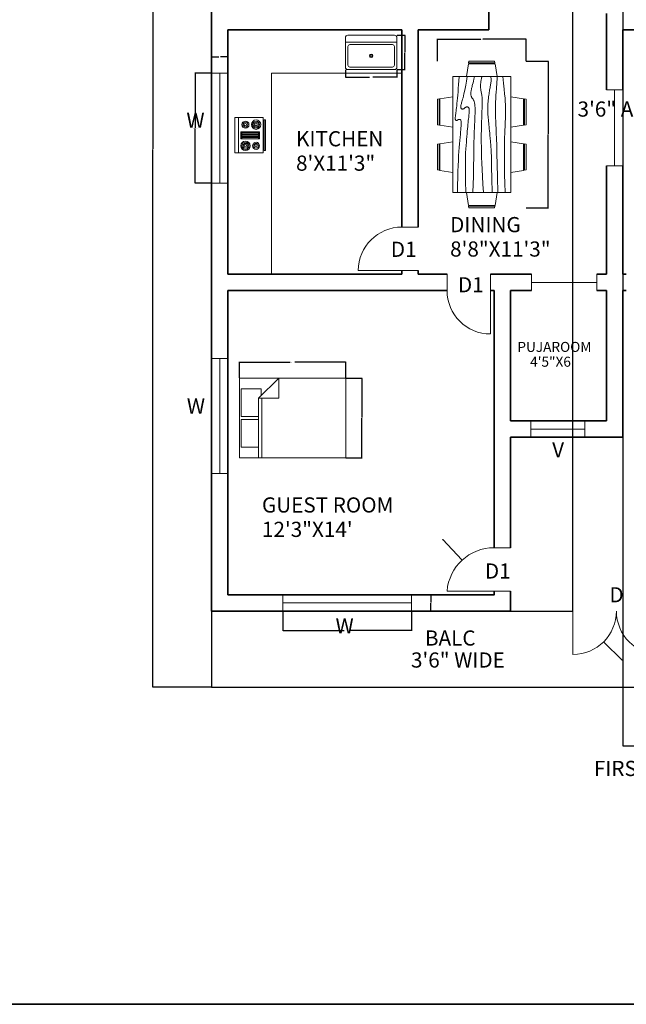
# Model space of a CAD drawing. Units: feet. Extents: x 1654 to 2985, y 1348 to 2230.
# Tile 41 of 53: x 2320 to 2655, y 1348 to 1892. Entities that reach past the tile are written whole.
import ezdxf

# ---------------------------------------------------------------- set-up
doc = ezdxf.new("R2010")
doc.units = ezdxf.units.FT
for name, color, linetype, lineweight in [('A-ANNO-DIMS', 2, 'Continuous', 18), ('A-ANNO-TEXT', 7, 'Continuous', 18), ('A-ANNO-TITL', 7, 'Continuous', 35), ('A-ANNO-TTLB', 7, 'Continuous', 35), ('A-AREA-IDEN', 7, 'Continuous', 18), ('A-DOOR', 3, 'Continuous', 18), ('A-EQPM', 9, 'Continuous', 18), ('A-FLOR', 7, 'Continuous', 25), ('A-FLOR-CASE', 8, 'Continuous', 18), ('A-FLOR-FIXT', 8, 'Continuous', 18), ('A-FURN', 8, 'Continuous', 13), ('A-GLAZ', 4, 'Continuous', 18), ('A-WALL', 7, 'Continuous', 35), ('A-WALL-OPEN', 4, 'Continuous', 18)]:
    doc.layers.add(name, color=color, linetype=linetype, lineweight=lineweight)
doc.styles.get("Standard").update_dxf_attribs({"font": 'arial.ttf'})
doc.dimstyles.get("Standard").update_dxf_attribs({"dimtxt": 0.18, "dimasz": 0.18, "dimexe": 0.18, "dimexo": 0.0625, "dimgap": 0.09, "dimtad": 0, "dimtih": 1, "dimtoh": 1, "dimdec": 4, "dimzin": 0, "dimdsep": 46, "dimtxsty": 'Standard', "dimcen": 0.09, "dimadec": 0, "dimazin": 0, "dimtfac": 1, "dimtdec": 4, "dimtofl": 0, "dimtmove": 0, "dimatfit": 3, "dimfxl": 1, "dimtolj": 1, "dimtzin": 0, "dimarcsym": 0})

# ---------------------------------------------------------------- blocks, each defined once
blk = doc.blocks.new('Dining Set - 36 x 72 in.')
for p, q in [((-22.2343, 26.00059), (-23.4847, 17.99762)), ((-22.2304, 26), (-5.7608, 26)), ((-22, 27.5), (-22.1562, 26.50042)), ((-5.8416, 26.5), (-22.1534, 26.5)), ((-22, 27.5), (-6, 27.5)), ((-5.8437, 26.49966), (-6, 27.5)), ((-4.5152, 17.99762), (-5.7655, 25.99926)), ((5.7657, 26.00059), (4.5153, 17.99762)), ((5.7696, 26), (22.2392, 26)), ((6, 27.5), (5.8438, 26.50042)), ((22.1584, 26.5), (5.8466, 26.5)), ((6, 27.5), (22, 27.5)), ((22.1563, 26.49966), (22, 27.5)), ((23.4848, 17.99762), (22.2345, 25.99926)), ((36, 18), (-36, 18)), ((-36, 18), (-36, -18)), ((36, -18), (36, 18)), ((-45.5, 8), (-44.5004, 8.15617)), ((-45.5, 8), (-45.5, -8)), ((-44.5, -8.15843), (-44.5, 8.15338)), ((-44.0006, 8.23428), (-35.9976, 9.48474)), ((-44, 8.23041), (-44, -8.23915)), ((44.0006, 8.23428), (35.9976, 9.48474)), ((44, 8.23041), (44, -8.23915)), ((44.5, -8.15843), (44.5, 8.15338)), ((45.5, 8), (44.5005, 8.15617)), ((45.5, 8), (45.5, -8)), ((-44.4997, -8.15631), (-45.5, -8)), ((-35.9976, -9.48476), (-43.9993, -8.2345)), ((35.9976, -9.48476), (43.9993, -8.2345)), ((44.4997, -8.15631), (45.5, -8)), ((-36, -18), (36, -18)), ((-22.2343, -26.0006), (-23.4847, -17.99762)), ((-4.5152, -17.99762), (-5.7655, -25.99928)), ((5.7657, -26.0006), (4.5153, -17.99762)), ((23.4848, -17.99762), (22.2345, -25.99928)), ((-22.2304, -26), (-5.7608, -26)), ((-22, -27.5), (-22.1562, -26.50044)), ((-5.8416, -26.5), (-22.1534, -26.5)), ((-22, -27.5), (-6, -27.5)), ((-5.8437, -26.49967), (-6, -27.5)), ((5.7696, -26), (22.2392, -26)), ((6, -27.5), (5.8438, -26.50044)), ((22.1584, -26.5), (5.8466, -26.5)), ((6, -27.5), (22, -27.5)), ((22.1563, -26.49967), (22, -27.5))]:
    blk.add_line(p, q)
for points in [[(-36, 15), (-31.1772, 14.97754), (-26.8079, 14.91406), (-22.8538, 14.81543), (-19.276, 14.6875), (-16.0362, 14.53613), (-13.0957, 14.36718), (-10.4159, 14.18652), (-7.9583, 14), (-5.6904, 13.81315), (-3.6035, 13.63021), (-1.6954, 13.45508), (0.0365, 13.29166), (1.5945, 13.14388), (2.9811, 13.01562), (4.1988, 12.9108), (5.25, 12.83333), (6.1393, 12.78613), (6.8802, 12.76823), (7.4883, 12.77767), (7.9792, 12.8125), (8.3685, 12.87077), (8.6719, 12.95052), (8.9049, 13.0498), (9.0833, 13.16666), (9.2205, 13.29899), (9.3216, 13.44401), (9.3895, 13.59879), (9.4271, 13.76041), (9.4373, 13.92594), (9.4232, 14.09245), (9.3875, 14.257), (9.3333, 14.41666), (9.2638, 14.56917), (9.1836, 14.71484), (9.0975, 14.85465), (9.0104, 14.98958), (8.9272, 15.1206), (8.8529, 15.2487), (8.7922, 15.37483), (8.75, 15.5), (8.7305, 15.62467), (8.7344, 15.74739), (8.7617, 15.86621), (8.8125, 15.97916), (8.8867, 16.08431), (8.9844, 16.17968), (9.1055, 16.26334), (9.25, 16.33333), (9.4189, 16.38802), (9.6172, 16.42708), (9.8506, 16.45052), (10.125, 16.45833), (10.4463, 16.45052), (10.8203, 16.42708), (11.2529, 16.38802), (11.75, 16.33333), (12.3184, 16.26318), (12.9694, 16.17838), (13.7151, 16.07991), (14.5677, 15.96875), (15.5395, 15.84586), (16.6426, 15.71224), (17.8893, 15.56884), (19.2917, 15.41666), (20.859, 15.25667), (22.5879, 15.08984), (24.4721, 14.91715), (26.5052, 14.73958), (28.6809, 14.5581), (30.9929, 14.3737), (33.4347, 14.18733), (36, 14)], [(-36, 10), (-28.9766, 10.14274), (-23.1725, 10.20442), (-18.4241, 10.19775), (-14.5677, 10.13541), (-11.4399, 10.03011), (-8.877, 9.89453), (-6.7154, 9.74137), (-4.7917, 9.58333), (-2.9698, 9.43082), (-1.2246, 9.28515), (0.4415, 9.14534), (2.026, 9.01041), (3.5266, 8.87939), (4.9408, 8.7513), (6.266, 8.62516), (7.5, 8.5), (8.6411, 8.37549), (9.6914, 8.2539), (10.6538, 8.13818), (11.5312, 8.03125), (12.3267, 7.93603), (13.043, 7.85547), (13.6831, 7.79248), (14.25, 7.75), (14.7471, 7.7303), (15.1797, 7.73307), (15.5537, 7.75732), (15.875, 7.80208), (16.1494, 7.86637), (16.3828, 7.94922), (16.5811, 8.04964), (16.75, 8.16666), (16.8944, 8.29915), (17.0143, 8.44531), (17.1089, 8.60319), (17.1771, 8.77083), (17.218, 8.94629), (17.2305, 9.1276), (17.2137, 9.31282), (17.1667, 9.5), (17.0895, 9.6875), (16.987, 9.875), (16.8649, 10.0625), (16.7292, 10.25), (16.5856, 10.4375), (16.4401, 10.625), (16.2985, 10.8125), (16.1667, 11), (16.05, 11.18733), (15.9518, 11.3737), (15.8752, 11.5581), (15.8229, 11.73958), (15.798, 11.91715), (15.8034, 12.08984), (15.842, 12.25667), (15.9167, 12.41666), (16.0295, 12.56836), (16.1784, 12.70833), (16.3605, 12.83268), (16.5729, 12.9375), (16.8127, 13.01888), (17.0768, 13.07291), (17.3625, 13.0957), (17.6667, 13.08333), (17.9894, 13.03312), (18.3418, 12.94726), (18.7382, 12.82918), (19.1927, 12.68229), (19.7195, 12.51001), (20.3327, 12.31575), (21.0465, 12.10294), (21.875, 11.875), (22.8357, 11.63354), (23.959, 11.37304), (25.2786, 11.08618), (26.8282, 10.76562), (28.6414, 10.40405), (30.752, 9.99414), (33.1936, 9.52856), (36, 9)], [(-36, 5.5), (-30.7157, 5.3348), (-26.069, 5.20963), (-21.9946, 5.11767), (-18.4271, 5.05208), (-15.3009, 5.00602), (-12.5508, 4.97265), (-10.1112, 4.94515), (-7.9167, 4.91666), (-5.909, 4.88167), (-4.0586, 4.83984), (-2.3429, 4.79215), (-0.7396, 4.73958), (0.7739, 4.6831), (2.22, 4.6237), (3.6213, 4.56233), (5, 4.5), (6.373, 4.43782), (7.7344, 4.3776), (9.0723, 4.32129), (10.375, 4.27083), (11.6309, 4.22819), (12.8281, 4.19531), (13.9551, 4.17415), (15, 4.16666), (15.954, 4.17448), (16.819, 4.19791), (17.6001, 4.23698), (18.3021, 4.29166), (18.9299, 4.36198), (19.4883, 4.44791), (19.9823, 4.54948), (20.4167, 4.66666), (20.7969, 4.79899), (21.1302, 4.94401), (21.4245, 5.09879), (21.6875, 5.26041), (21.9271, 5.42594), (22.1511, 5.59245), (22.3672, 5.757), (22.5834, 5.91666), (22.8065, 6.06868), (23.0404, 6.21093), (23.2879, 6.34147), (23.5521, 6.45833), (23.8358, 6.55957), (24.142, 6.64323), (24.4735, 6.70735), (24.8334, 6.75), (25.2235, 6.76969), (25.642, 6.76692), (26.0858, 6.74267), (26.5521, 6.69791), (27.0379, 6.63362), (27.5404, 6.55078), (28.0565, 6.45036), (28.5834, 6.33333), (29.1242, 6.19987), (29.7071, 6.04687), (30.3661, 5.87044), (31.1354, 5.66666), (32.0493, 5.43164), (33.142, 5.16146), (34.4475, 4.85221), (36, 4.5)], [(-36, -1), (-30.7915, -0.6591), (-26.0195, -0.38216), (-21.6519, -0.16284), (-17.6563, 0.00521), (-14.0005, 0.12833), (-10.6523, 0.21289), (-7.5796, 0.26522), (-4.75, 0.29166), (-2.134, 0.29793), (0.2878, 0.28711), (2.5317, 0.26163), (4.6146, 0.22396), (6.5529, 0.17651), (8.3633, 0.12174), (10.0623, 0.06209), (11.6667, 0), (13.1899, -0.06201), (14.6341, -0.1211), (15.9982, -0.17432), (17.2813, -0.21875), (18.4823, -0.25147), (19.6003, -0.26953), (20.6343, -0.27002), (21.5834, -0.25), (22.4481, -0.20768), (23.2357, -0.14584), (23.9549, -0.06836), (24.6146, 0.02083), (25.2235, 0.11784), (25.7904, 0.21875), (26.3241, 0.31966), (26.8334, 0.41666), (27.3265, 0.50618), (27.8099, 0.58593), (28.2894, 0.65397), (28.7709, 0.70833), (29.2601, 0.74707), (29.763, 0.76823), (30.2855, 0.76985), (30.8334, 0.75), (31.4088, 0.70784), (31.9994, 0.64713), (32.589, 0.57275), (33.1615, 0.48958), (33.7008, 0.4025), (34.1908, 0.3164), (34.6153, 0.23616), (34.9584, 0.16666), (35.2099, 0.11165), (35.3848, 0.07031), (35.504, 0.04069), (35.5886, 0.02083), (35.6594, 0.00879), (35.7377, 0.0026), (35.8442, 0.00032), (36, 0)], [(-36, -6.5), (-27.1843, -6.31267), (-20.084, -6.1263), (-14.469, -5.9419), (-10.1094, -5.76042), (-6.7752, -5.58285), (-4.2363, -5.41016), (-2.2629, -5.24333), (-0.625, -5.08334), (0.8708, -4.93099), (2.2715, -4.78646), (3.5872, -4.64974), (4.8281, -4.52084), (6.0046, -4.39974), (7.127, -4.28646), (8.2053, -4.18099), (9.25, -4.08334), (10.2705, -3.99382), (11.2734, -3.91407), (12.2647, -3.84603), (13.25, -3.79167), (14.2354, -3.75293), (15.2266, -3.73177), (16.2295, -3.73015), (17.25, -3.75), (18.2912, -3.79248), (19.3451, -3.85547), (20.4009, -3.93604), (21.4479, -4.03125), (22.4754, -4.13819), (23.4727, -4.25391), (24.4289, -4.37549), (25.3334, -4.5), (26.1785, -4.62492), (26.9694, -4.74935), (27.7145, -4.87281), (28.4219, -4.99479), (29.1, -5.11483), (29.7572, -5.23242), (30.4016, -5.34709), (31.0417, -5.45834), (31.6837, -5.56437), (32.3262, -5.65821), (32.9658, -5.73153), (33.599, -5.77604), (34.2224, -5.78345), (34.8327, -5.74545), (35.4264, -5.65373), (36, -5.5)], [(-36, -10), (-26.4022, -9.81299), (-18.4675, -9.62891), (-11.9839, -9.45069), (-6.7396, -9.28125), (-2.5226, -9.12354), (0.8789, -8.98047), (3.6769, -8.85498), (6.0833, -8.75), (8.2767, -8.66765), (10.3021, -8.60677), (12.1712, -8.56543), (13.8958, -8.54167), (15.4876, -8.53353), (16.9583, -8.53907), (18.3197, -8.55632), (19.5834, -8.58334), (20.7616, -8.61841), (21.8685, -8.66081), (22.9188, -8.71004), (23.9271, -8.76563), (24.9081, -8.82707), (25.8763, -8.89388), (26.8465, -8.96558), (27.8334, -9.04167), (28.8474, -9.12118), (29.8828, -9.20117), (30.93, -9.27824), (31.9792, -9.34896), (33.0205, -9.40991), (34.0443, -9.45768), (35.0407, -9.48885), (36, -9.5)], [(-36, -14.5), (-30.0881, -14.33513), (-25.0332, -14.21224), (-20.7312, -14.12647), (-17.0781, -14.07292), (-13.97, -14.04671), (-11.3027, -14.04297), (-8.9724, -14.05681), (-6.875, -14.08334), (-4.9224, -14.11833), (-3.0905, -14.16016), (-1.3709, -14.20785), (0.2448, -14.26042), (1.7647, -14.3169), (3.1973, -14.3763), (4.5507, -14.43767), (5.8333, -14.5), (7.0554, -14.5621), (8.235, -14.62175), (9.3922, -14.67652), (10.5469, -14.72396), (11.7192, -14.76164), (12.929, -14.78711), (14.1965, -14.79794), (15.5417, -14.79167), (16.9933, -14.76424), (18.6152, -14.70508), (20.4804, -14.60197), (22.6615, -14.44271), (25.2312, -14.21509), (28.2624, -13.9069), (31.8277, -13.50594), (36, -13)]]:
    blk.add_lwpolyline(points)
blk = doc.blocks.new('Range-Oven - 30 in top')
for p, q in [((0, -3), (30, -3)), ((12, -6), (18, -6)), ((13, -20), (13, -6)), ((14, -6), (14, -20)), ((15, -20), (15, -6)), ((16, -6), (16, -20)), ((17, -20), (17, -6)), ((6, -24), (6, -25)), ((8, -25), (8, -24)), ((18, -20), (12, -20)), ((22, -25), (22, -24)), ((24, -24), (24, -25))]:
    blk.add_line(p, q)
for points in [[(0, -24), (0, 0), (30, 0), (30, -24)], [(12, -21), (12, -5), (18, -5), (18, -21)], [(2, -26), (2, -25), (28, -25), (28, -26)]]:
    blk.add_lwpolyline(points, close=True)
for centre, radius in [((6, -9), 4), ((6, -9), 3), ((6, -9), 2), ((6, -9), 1), ((24, -9), 3), ((24, -9), 2), ((24, -9), 1), ((6, -18), 3), ((6, -18), 2), ((24, -18), 4), ((24, -18), 3), ((24, -18), 2), ((6, -18), 1), ((24, -18), 1)]:
    blk.add_circle(centre, radius)
blk = doc.blocks.new('Sink-single - 30 in top')
blk.add_line((-15, -3.999996), (15, -3.999996))
for points in [[(-13.5, 0), (13.5, 0)], [(-15, -18.499996), (-15, -1.5)], [(-12.5, -5.499996), (12.5, -5.499996)], [(15, -1.5), (15, -18.499996)], [(-13.5, -17.499996), (-13.5, -6.499996)], [(13.5, -6.499996), (13.5, -17.499996)], [(13.5, -19.999996), (-13.5, -19.999996)], [(12.5, -18.499996), (-12.5, -18.499996)]]:
    blk.add_lwpolyline(points)
for radius in [1, 0.5]:
    blk.add_circle((0, -11.999996), radius)
for centre, radius, start, end in [((-13.5, -1.5), 1.5, 90, 180), ((-12.5, -6.499996), 1, 90, 180), ((12.5, -6.499996), 1, 0, 90), ((13.5, -1.5), 1.5, 0, 90), ((-13.5, -18.499996), 1.5, 180, 270), ((-12.5, -17.499996), 1, 180, 270), ((12.5, -17.499996), 1, 270, 0), ((13.5, -18.499996), 1.5, 270, 0)]:
    blk.add_arc(centre, radius, start, end)
blk = doc.blocks.new('Bed - Queen')
for p, q in [((0, -80.00003), (0, 0)), ((0, 0), (59.99999, 0)), ((59.99999, 0), (59.99999, -80.00003)), ((7.99999, -1.2), (28.79998, -1.2)), ((7.99999, -14.4), (7.99999, -1.2)), ((28.79998, -1.2), (28.79998, -14.4)), ((31.19999, -1.2), (51.99999, -1.2)), ((31.19999, -14.4), (31.19999, -1.2)), ((51.99999, -1.2), (51.99999, -16.4)), ((0, -14.4), (44.8, -14.4)), ((59.99999, -29.6), (44.8, -14.4)), ((44.8, -14.4), (44.8, -29.6)), ((44.8, -16.8), (0, -16.8)), ((51.99999, -16.4), (46.79936, -16.4)), ((44.8, -29.6), (59.99999, -29.6)), ((59.99999, -80.00003), (0, -80.00003))]:
    blk.add_line(p, q)
blk = doc.blocks.new('DOOR-INT-SINGLE')
for p, q in [((0, 24), (9, 24)), ((-24, 0), (9, 0))]:
    blk.add_line(p, q)
blk.add_arc((0, 0), 24, 90, 180)
blk = doc.blocks.new('DOOR-GUEST-ENTRY')
for p, q in [((-2, 26.08), (9, 26.08)), ((-26, 2.08), (9, 2.08))]:
    blk.add_line(p, q)
blk.add_arc((0, 0), 26.08, 90, 175.4188)
blk = doc.blocks.new('WIN-KITCHEN')
for p, q in [((0, 60.69), (9, 60.69)), ((4.5, 60.69), (4.5, 0)), ((0, 0), (9, 0))]:
    blk.add_line(p, q)
blk = doc.blocks.new('WIN-GUEST-SIDE')
for p, q in [((0, 63.53), (9, 63.53)), ((4.5, 63.53), (4.5, 0)), ((9, 0), (0, 0))]:
    blk.add_line(p, q)
blk = doc.blocks.new('WIN-GUEST-FRONT')
for p, q in [((0, 9), (0, 0)), ((71.09, 9), (71.09, 0)), ((0, 4.5), (71.09, 4.5))]:
    blk.add_line(p, q)
blk = doc.blocks.new('OPENING-PUJA')
for p, q in [((0, 9), (0, 0)), ((36, 9), (36, 0)), ((0, 4.5), (36, 4.5))]:
    blk.add_line(p, q)
blk = doc.blocks.new('OPENING-LIVING-ARCH')
for p, q in [((0, 42), (9, 42)), ((4.5, 42), (4.5, 0)), ((9, 0), (0, 0))]:
    blk.add_line(p, q)
blk = doc.blocks.new('CASEWORK-KITCHEN-L')
for q in [(72, 111), (0, 0)]:
    blk.add_line((0, 111), q)
blk = doc.blocks.new('*D36')
at = {"layer": 'A-ANNO-DIMS', "color": 0, "lineweight": -2, "transparency": 16777216}
for p, q in [((2441.06, 1693.97), (2441.06, 1702.9)), ((2441.24, 1702.72), (2469.12, 1702.72)), ((2499.6, 1702.72), (2471.72, 1702.72)), ((2499.78, 1693.97), (2499.78, 1702.9))]:
    blk.add_line(p, q, dxfattribs=at)
at = {"layer": 'A-ANNO-DIMS', "color": 0, "transparency": 16777216}
for points in [[(2441.24, 1702.75), (2441.24, 1702.69), (2441.06, 1702.72)], [(2499.6, 1702.75), (2499.6, 1702.69), (2499.78, 1702.72)]]:
    blk.add_solid(points, dxfattribs=at)
at = {"layer": 'Defpoints', "color": 0, "transparency": 16777216}
for p in [(2441.06, 1702.72), (2441.06, 1693.91), (2499.78, 1693.91)]:
    blk.add_point(p, dxfattribs=at)
at = {"layer": 'A-ANNO-DIMS', "color": 0, "transparency": 16777216, "insert": (2470.42, 1702.72), "char_height": 0.18, "attachment_point": 5}
blk.add_mtext('\\A1;QUEEN BED 59 TYP.', dxfattribs=at)
blk = doc.blocks.new('*D37')
at = {"layer": 'A-ANNO-DIMS', "color": 0, "lineweight": -2, "transparency": 16777216}
for p, q in [((2499.84, 1693.91), (2508.76, 1693.91)), ((2508.58, 1693.73), (2508.58, 1672.07)), ((2508.58, 1650.06), (2508.58, 1671.71)), ((2499.84, 1649.88), (2508.76, 1649.88))]:
    blk.add_line(p, q, dxfattribs=at)
at = {"layer": 'A-ANNO-DIMS', "color": 0, "transparency": 16777216}
for points in [[(2508.55, 1693.73), (2508.61, 1693.73), (2508.58, 1693.91)], [(2508.55, 1650.06), (2508.61, 1650.06), (2508.58, 1649.88)]]:
    blk.add_solid(points, dxfattribs=at)
at = {"layer": 'Defpoints', "color": 0, "transparency": 16777216}
for p in [(2499.78, 1693.91), (2508.58, 1693.91), (2499.78, 1649.88)]:
    blk.add_point(p, dxfattribs=at)
at = {"layer": 'A-ANNO-DIMS', "color": 0, "transparency": 16777216, "insert": (2508.58, 1671.89), "char_height": 0.18, "attachment_point": 5}
blk.add_mtext('\\A1;44 TYP.', dxfattribs=at)
blk = doc.blocks.new('*D42')
at = {"layer": 'A-ANNO-DIMS', "color": 0, "lineweight": -2, "transparency": 16777216}
for p, q in [((2599.4, 1868.82), (2611.66, 1868.82)), ((2611.48, 1868.64), (2611.48, 1828.54)), ((2611.48, 1788.07), (2611.48, 1828.17)), ((2599.4, 1787.89), (2611.66, 1787.89))]:
    blk.add_line(p, q, dxfattribs=at)
at = {"layer": 'A-ANNO-DIMS', "color": 0, "transparency": 16777216}
for points in [[(2611.45, 1868.64), (2611.51, 1868.64), (2611.48, 1868.82)], [(2611.45, 1788.07), (2611.51, 1788.07), (2611.48, 1787.89)]]:
    blk.add_solid(points, dxfattribs=at)
at = {"layer": 'Defpoints', "color": 0, "transparency": 16777216}
for p in [(2599.34, 1868.82), (2611.48, 1868.82), (2599.34, 1787.89)]:
    blk.add_point(p, dxfattribs=at)
at = {"layer": 'A-ANNO-DIMS', "color": 0, "transparency": 16777216, "insert": (2611.48, 1828.35), "char_height": 0.18, "attachment_point": 5}
blk.add_mtext('\\A1;DINING SET 81 TYP.', dxfattribs=at)
blk = doc.blocks.new('*D43')
at = {"layer": 'A-ANNO-DIMS', "color": 0, "lineweight": -2, "transparency": 16777216}
for p, q in [((2550.42, 1868.88), (2550.42, 1881.14)), ((2599.34, 1868.88), (2599.34, 1881.14)), ((2550.6, 1880.96), (2574.35, 1880.96)), ((2599.16, 1880.96), (2575.41, 1880.96))]:
    blk.add_line(p, q, dxfattribs=at)
at = {"layer": 'A-ANNO-DIMS', "color": 0, "transparency": 16777216}
for points in [[(2550.6, 1880.99), (2550.6, 1880.93), (2550.42, 1880.96)], [(2599.16, 1880.99), (2599.16, 1880.93), (2599.34, 1880.96)]]:
    blk.add_solid(points, dxfattribs=at)
at = {"layer": 'Defpoints', "color": 0, "transparency": 16777216}
for p in [(2550.42, 1880.96), (2550.42, 1868.82), (2599.34, 1868.82)]:
    blk.add_point(p, dxfattribs=at)
at = {"layer": 'A-ANNO-DIMS', "color": 0, "transparency": 16777216, "insert": (2574.88, 1880.96), "char_height": 0.18, "attachment_point": 5}
blk.add_mtext('\\A1;49 TYP.', dxfattribs=at)
blk = doc.blocks.new('*D46')
at = {"layer": 'A-ANNO-DIMS', "color": 0, "lineweight": -2, "transparency": 16777216}
for p, q in [((2499.55, 1864.16), (2499.55, 1859.77)), ((2499.73, 1859.95), (2512.94, 1859.95)), ((2527.86, 1859.95), (2514.65, 1859.95)), ((2528.04, 1864.16), (2528.04, 1859.77))]:
    blk.add_line(p, q, dxfattribs=at)
at = {"layer": 'A-ANNO-DIMS', "color": 0, "transparency": 16777216}
for points in [[(2499.73, 1859.98), (2499.73, 1859.92), (2499.55, 1859.95)], [(2527.86, 1859.98), (2527.86, 1859.92), (2528.04, 1859.95)]]:
    blk.add_solid(points, dxfattribs=at)
at = {"layer": 'Defpoints', "color": 0, "transparency": 16777216}
for p in [(2499.55, 1864.22), (2528.04, 1864.22), (2528.04, 1859.95)]:
    blk.add_point(p, dxfattribs=at)
at = {"layer": 'A-ANNO-DIMS', "color": 0, "transparency": 16777216, "insert": (2513.79, 1859.95), "char_height": 0.18, "attachment_point": 5}
blk.add_mtext('\\A1;SINK 28 TYP.', dxfattribs=at)
blk = doc.blocks.new('*D47')
at = {"layer": 'A-ANNO-DIMS', "color": 0, "lineweight": -2, "transparency": 16777216}
for p, q in [((2528.1, 1883.21), (2532.49, 1883.21)), ((2532.31, 1883.03), (2532.31, 1873.9)), ((2532.31, 1864.4), (2532.31, 1873.54)), ((2528.1, 1864.22), (2532.49, 1864.22))]:
    blk.add_line(p, q, dxfattribs=at)
at = {"layer": 'A-ANNO-DIMS', "color": 0, "transparency": 16777216}
for points in [[(2532.28, 1883.03), (2532.34, 1883.03), (2532.31, 1883.21)], [(2532.28, 1864.4), (2532.34, 1864.4), (2532.31, 1864.22)]]:
    blk.add_solid(points, dxfattribs=at)
at = {"layer": 'Defpoints', "color": 0, "transparency": 16777216}
for p in [(2528.04, 1883.21), (2532.31, 1883.21), (2528.04, 1864.22)]:
    blk.add_point(p, dxfattribs=at)
at = {"layer": 'A-ANNO-DIMS', "color": 0, "transparency": 16777216, "insert": (2532.31, 1873.72), "char_height": 0.18, "attachment_point": 5}
blk.add_mtext('\\A1;19 TYP.', dxfattribs=at)
blk = doc.blocks.new('*D60')
at = {"layer": 'A-ANNO-DIMS', "color": 0, "lineweight": -2, "transparency": 16777216}
for p, q in [((2425.64, 1862.16), (2416.42, 1862.16)), ((2416.6, 1861.98), (2416.6, 1832)), ((2416.6, 1801.65), (2416.6, 1831.63)), ((2425.64, 1801.47), (2416.42, 1801.47))]:
    blk.add_line(p, q, dxfattribs=at)
at = {"layer": 'A-ANNO-DIMS', "color": 0, "transparency": 16777216}
for points in [[(2416.57, 1861.98), (2416.63, 1861.98), (2416.6, 1862.16)], [(2416.57, 1801.65), (2416.63, 1801.65), (2416.6, 1801.47)]]:
    blk.add_solid(points, dxfattribs=at)
at = {"layer": 'Defpoints', "color": 0, "transparency": 16777216}
for p in [(2425.71, 1862.16), (2416.6, 1801.47), (2425.71, 1801.47)]:
    blk.add_point(p, dxfattribs=at)
at = {"layer": 'A-ANNO-DIMS', "color": 0, "transparency": 16777216, "insert": (2416.6, 1831.81), "char_height": 0.18, "attachment_point": 5}
blk.add_mtext('\\A1;KITCHEN WIN. 61 TYP.', dxfattribs=at)
blk = doc.blocks.new('*D61')
at = {"layer": 'A-ANNO-DIMS', "color": 0, "lineweight": -2, "transparency": 16777216}
for p, q in [((2425.71, 1862.22), (2425.71, 1871.44)), ((2425.89, 1871.26), (2429.75, 1871.26)), ((2434.53, 1871.26), (2430.66, 1871.26)), ((2434.71, 1862.22), (2434.71, 1871.44))]:
    blk.add_line(p, q, dxfattribs=at)
at = {"layer": 'A-ANNO-DIMS', "color": 0, "transparency": 16777216}
for points in [[(2425.89, 1871.29), (2425.89, 1871.23), (2425.71, 1871.26)], [(2434.53, 1871.29), (2434.53, 1871.23), (2434.71, 1871.26)]]:
    blk.add_solid(points, dxfattribs=at)
at = {"layer": 'Defpoints', "color": 0, "transparency": 16777216}
for p in [(2425.71, 1871.26), (2425.71, 1862.16), (2434.71, 1862.16)]:
    blk.add_point(p, dxfattribs=at)
at = {"layer": 'A-ANNO-DIMS', "color": 0, "transparency": 16777216, "insert": (2430.21, 1871.26), "char_height": 0.18, "attachment_point": 5}
blk.add_mtext('\\A1;9 TYP.', dxfattribs=at)
blk = doc.blocks.new('*D66')
at = {"layer": 'A-ANNO-DIMS', "color": 0, "lineweight": -2, "transparency": 16777216}
for p, q in [((2465, 1565.19), (2465, 1554.41)), ((2536.08, 1565.19), (2536.08, 1554.41)), ((2465.18, 1554.59), (2498.96, 1554.59)), ((2535.9, 1554.59), (2502.12, 1554.59))]:
    blk.add_line(p, q, dxfattribs=at)
at = {"layer": 'A-ANNO-DIMS', "color": 0, "transparency": 16777216}
for points in [[(2465.18, 1554.62), (2465.18, 1554.56), (2465, 1554.59)], [(2535.9, 1554.62), (2535.9, 1554.56), (2536.08, 1554.59)]]:
    blk.add_solid(points, dxfattribs=at)
at = {"layer": 'Defpoints', "color": 0, "transparency": 16777216}
for p in [(2465, 1565.25), (2536.08, 1565.25), (2536.08, 1554.59)]:
    blk.add_point(p, dxfattribs=at)
at = {"layer": 'A-ANNO-DIMS', "color": 0, "transparency": 16777216, "insert": (2500.54, 1554.59), "char_height": 0.18, "attachment_point": 5}
blk.add_mtext('\\A1;FRONT WINDOW 71 TYP.', dxfattribs=at)
blk = doc.blocks.new('*D67')
at = {"layer": 'A-ANNO-DIMS', "color": 0, "lineweight": -2, "transparency": 16777216}
for p, q in [((2536.15, 1574.25), (2546.93, 1574.25)), ((2546.75, 1574.07), (2546.75, 1569.94)), ((2546.75, 1565.43), (2546.75, 1569.57)), ((2536.15, 1565.25), (2546.93, 1565.25))]:
    blk.add_line(p, q, dxfattribs=at)
at = {"layer": 'A-ANNO-DIMS', "color": 0, "transparency": 16777216}
for points in [[(2546.72, 1574.07), (2546.78, 1574.07), (2546.75, 1574.25)], [(2546.72, 1565.43), (2546.78, 1565.43), (2546.75, 1565.25)]]:
    blk.add_solid(points, dxfattribs=at)
at = {"layer": 'Defpoints', "color": 0, "transparency": 16777216}
for p in [(2536.08, 1574.25), (2546.75, 1574.25), (2536.08, 1565.25)]:
    blk.add_point(p, dxfattribs=at)
at = {"layer": 'A-ANNO-DIMS', "color": 0, "transparency": 16777216, "insert": (2546.75, 1569.75), "char_height": 0.18, "attachment_point": 5}
blk.add_mtext('\\A1;9 TYP.', dxfattribs=at)
blk = doc.blocks.new('*D79')
at = {"layer": 'A-ANNO-DIMS', "color": 0, "lineweight": -2, "transparency": 16777216}
for p, q in [((2425.64, 2117.25), (2393.08, 2117.25)), ((2393.26, 2117.07), (2393.26, 1820.44)), ((2393.26, 1523.43), (2393.26, 1820.07)), ((2425.64, 1523.25), (2393.08, 1523.25))]:
    blk.add_line(p, q, dxfattribs=at)
at = {"layer": 'A-ANNO-DIMS', "color": 0, "transparency": 16777216}
for points in [[(2393.23, 2117.07), (2393.29, 2117.07), (2393.26, 2117.25)], [(2393.23, 1523.43), (2393.29, 1523.43), (2393.26, 1523.25)]]:
    blk.add_solid(points, dxfattribs=at)
at = {"layer": 'Defpoints', "color": 0, "transparency": 16777216}
for p in [(2393.26, 2117.25), (2425.71, 2117.25), (2425.71, 1523.25)]:
    blk.add_point(p, dxfattribs=at)
at = {"layer": 'A-ANNO-DIMS', "color": 0, "transparency": 16777216, "insert": (2393.26, 1820.25), "char_height": 0.18, "attachment_point": 5}
blk.add_mtext('\\A1;594', dxfattribs=at)
blk = doc.blocks.new('*D82')
at = {"layer": 'A-ANNO-DIMS', "color": 0, "lineweight": -2, "transparency": 16777216}
for p, q in [((2652.71, 2039.19), (2652.71, 1490.62)), ((2784.71, 2039.19), (2784.71, 1490.62)), ((2652.89, 1490.8), (2718.43, 1490.8)), ((2784.53, 1490.8), (2718.99, 1490.8))]:
    blk.add_line(p, q, dxfattribs=at)
at = {"layer": 'A-ANNO-DIMS', "color": 0, "transparency": 16777216}
for points in [[(2652.89, 1490.83), (2652.89, 1490.77), (2652.71, 1490.8)], [(2784.53, 1490.83), (2784.53, 1490.77), (2784.71, 1490.8)]]:
    blk.add_solid(points, dxfattribs=at)
at = {"layer": 'Defpoints', "color": 0, "transparency": 16777216}
for p in [(2652.71, 2039.25), (2784.71, 2039.25), (2784.71, 1490.8)]:
    blk.add_point(p, dxfattribs=at)
at = {"layer": 'A-ANNO-DIMS', "color": 0, "transparency": 16777216, "insert": (2718.71, 1490.8), "char_height": 0.18, "attachment_point": 5}
blk.add_mtext('\\A1;132', dxfattribs=at)
blk = doc.blocks.new('*D84')
at = {"layer": 'A-ANNO-DIMS', "color": 0, "lineweight": -2, "transparency": 16777216}
for p, q in [((2625.24, 1565.32), (2625.24, 2149.88)), ((2625.42, 2149.7), (2649.01, 2149.7)), ((2673.06, 2149.7), (2649.46, 2149.7)), ((2673.24, 1565.32), (2673.24, 2149.88))]:
    blk.add_line(p, q, dxfattribs=at)
at = {"layer": 'A-ANNO-DIMS', "color": 0, "transparency": 16777216}
for points in [[(2625.42, 2149.73), (2625.42, 2149.67), (2625.24, 2149.7)], [(2673.06, 2149.73), (2673.06, 2149.67), (2673.24, 2149.7)]]:
    blk.add_solid(points, dxfattribs=at)
at = {"layer": 'Defpoints', "color": 0, "transparency": 16777216}
for p in [(2673.24, 2149.7), (2625.24, 1565.25), (2673.24, 1565.25)]:
    blk.add_point(p, dxfattribs=at)
at = {"layer": 'A-ANNO-DIMS', "color": 0, "transparency": 16777216, "insert": (2649.24, 2149.7), "char_height": 0.18, "attachment_point": 5}
blk.add_mtext('\\A1;48', dxfattribs=at)
blk = doc.blocks.new('*D106')
at = {"layer": 'A-ANNO-DIMS', "color": 0, "lineweight": -2, "transparency": 16777216}
for p, q in [((2625.15, 1565.25), (2625.33, 1565.25)), ((2625.24, 1565.16), (2625.24, 1565.34)), ((2652.39, 1538.1), (2642.33, 1548.16)), ((2652.57, 1538.1), (2652.39, 1538.1))]:
    blk.add_line(p, q, dxfattribs=at)
at = {"layer": 'A-ANNO-DIMS', "color": 0, "transparency": 16777216}
blk.add_solid([(2642.35, 1548.18), (2642.31, 1548.14), (2642.21, 1548.28)], dxfattribs=at)
at = {"layer": 'Defpoints', "color": 0, "transparency": 16777216}
for p in [(2625.24, 1565.25), (2642.21, 1548.28)]:
    blk.add_point(p, dxfattribs=at)
at = {"layer": 'A-ANNO-DIMS', "color": 0, "transparency": 16777216, "insert": (2653.07, 1538.1), "char_height": 0.18, "attachment_point": 5}
blk.add_mtext('\\A1;9X R24', dxfattribs=at)
blk = doc.blocks.new('*D107')
at = {"layer": 'A-ANNO-DIMS', "color": 0, "lineweight": -2, "transparency": 16777216}
for p, q in [((2553.22, 1604.84), (2553.4, 1604.84)), ((2553.4, 1604.84), (2563.89, 1593.47)), ((2581.62, 1574.17), (2581.8, 1574.17)), ((2581.71, 1574.08), (2581.71, 1574.26))]:
    blk.add_line(p, q, dxfattribs=at)
at = {"layer": 'A-ANNO-DIMS', "color": 0, "transparency": 16777216}
blk.add_solid([(2563.91, 1593.49), (2563.87, 1593.45), (2564.01, 1593.34)], dxfattribs=at)
at = {"layer": 'Defpoints', "color": 0, "transparency": 16777216}
for p in [(2564.01, 1593.34), (2581.71, 1574.17)]:
    blk.add_point(p, dxfattribs=at)
at = {"layer": 'A-ANNO-DIMS', "color": 0, "transparency": 16777216, "insert": (2552.67, 1604.84), "char_height": 0.18, "attachment_point": 5}
blk.add_mtext('\\A1;R26.083', dxfattribs=at)

msp = doc.modelspace()

# ---------------------------------------------------------------- linework, layer by layer
at = {"layer": 'A-ANNO-TTLB'}
msp.add_lwpolyline([(1654.1997, 2230.0267), (2985.175, 2230.0267), (2985.175, 1348.1324), (1654.1997, 1348.1324)], close=True, dxfattribs=at)
at = {"layer": 'A-DOOR'}
msp.add_line((2625.2353, 1565.2549), (2625.2353, 1541.2549), dxfattribs=at)
for centre, start, end in [((2625.2353, 1565.2549), 270, 0), ((2673.2353, 1565.2549), 180, 270)]:
    msp.add_arc(centre, 24, start, end, dxfattribs=at)
at = {"layer": 'A-FLOR'}
for p, q in [((2425.7058, 1565.2549), (2425.7058, 1523.2549)), ((2590.7058, 1565.2549), (2625.2353, 1565.2549)), ((2425.7058, 1523.2549), (2793.7058, 1523.2549))]:
    msp.add_line(p, q, dxfattribs=at)
at = {"layer": 'A-GLAZ'}
for p, q in [((2602.0206, 1670.2549), (2602.0206, 1661.2549)), ((2631.7283, 1670.2549), (2631.7283, 1661.2549)), ((2602.0206, 1665.7549), (2631.7283, 1665.7549))]:
    msp.add_line(p, q, dxfattribs=at)
at = {"layer": 'A-WALL'}
for p, q in [((2425.7058, 2117.2549), (2425.7058, 1565.2549)), ((2578.7058, 1886.2549), (2578.7058, 1897.2549)), ((2643.7058, 1895.2549), (2643.7058, 1886.2549)), ((2425.7058, 1886.2549), (2425.7058, 1751.2549)), ((2434.7058, 1886.2549), (2530.7058, 1886.2549)), ((2434.7058, 1886.2549), (2434.7058, 1751.2549)), ((2530.7058, 1777.2549), (2530.7058, 1886.2549)), ((2539.7058, 1886.2549), (2578.7058, 1886.2549)), ((2539.7058, 1777.2549), (2539.7058, 1886.2549)), ((2643.7058, 1853.0815), (2643.7058, 1886.2549)), ((2784.7058, 1886.2549), (2652.7058, 1886.2549)), ((2652.7058, 1853.0815), (2652.7058, 1886.2549)), ((2643.7058, 1751.2549), (2643.7058, 1811.0815)), ((2652.7058, 1751.2549), (2652.7058, 1811.0815)), ((2434.7058, 1751.2549), (2530.7058, 1751.2549)), ((2530.7058, 1751.2549), (2530.7058, 1753.2549)), ((2539.7058, 1751.2549), (2539.7058, 1753.2549)), ((2555.7058, 1751.2549), (2539.7058, 1751.2549)), ((2581.7058, 1751.2549), (2579.7058, 1751.2549)), ((2602.3701, 1751.2549), (2579.7058, 1751.2549)), ((2643.7058, 1751.2549), (2638.3701, 1751.2549)), ((2654.7058, 1751.2549), (2652.7058, 1751.2549)), ((2425.7058, 1742.2549), (2425.7058, 1565.2549)), ((2434.7058, 1742.2549), (2530.7058, 1742.2549)), ((2434.7058, 1742.2549), (2434.7058, 1574.2549)), ((2555.7058, 1742.2549), (2530.7058, 1742.2549)), ((2581.7058, 1742.2549), (2579.7058, 1742.2549)), ((2581.7058, 1600.2549), (2581.7058, 1742.2549)), ((2590.7058, 1670.2549), (2590.7058, 1742.2549)), ((2590.7058, 1742.2549), (2602.3701, 1742.2549)), ((2638.3701, 1742.2549), (2643.7058, 1742.2549)), ((2643.7058, 1742.2549), (2643.7058, 1670.2549)), ((2654.7058, 1742.2549), (2652.7058, 1742.2549)), ((2652.7058, 1742.2549), (2652.7058, 1661.2549)), ((2643.7058, 1670.2549), (2590.7058, 1670.2549)), ((2590.7058, 1600.2549), (2590.7058, 1661.2549)), ((2652.7058, 1661.2549), (2590.7058, 1661.2549)), ((2434.7058, 1574.2549), (2581.7058, 1574.2549)), ((2581.7058, 1574.2549), (2581.7058, 1576.2549)), ((2590.7058, 1565.2549), (2590.7058, 1576.2549)), ((2425.7058, 1565.2549), (2590.7058, 1565.2549))]:
    msp.add_line(p, q, dxfattribs=at)

# ---------------------------------------------------------------- block references
at = {"layer": 'A-DOOR'}
for name, p in [('DOOR-INT-SINGLE', (2530.7058, 1753.2549)), ('DOOR-GUEST-ENTRY', (2581.7058, 1574.1716))]:
    msp.add_blockref(name, p, dxfattribs=at)
at = {"layer": 'A-DOOR', "rotation": 90.00000000000003}
msp.add_blockref('DOOR-INT-SINGLE', (2579.7058, 1742.2549), dxfattribs=at)
at = {"layer": 'A-EQPM', "xscale": 0.6488816563275249, "yscale": 0.6488816563275249, "zscale": 0.6488816563275249, "rotation": 90}
msp.add_blockref('Range-Oven - 30 in top', (2438.5382, 1818.2456), dxfattribs=at)
at = {"layer": 'A-FLOR-CASE'}
msp.add_blockref('CASEWORK-KITCHEN-L', (2458.7054, 1751.255), dxfattribs=at)
at = {"layer": 'A-FLOR-FIXT', "xscale": 0.9494788357391524, "yscale": 0.9494788357391524, "zscale": 0.9494788357391524}
msp.add_blockref('Sink-single - 30 in top', (2513.7944, 1883.2123), dxfattribs=at)
at = {"layer": 'A-FURN', "rotation": 90}
for name, p, xscale, yscale, zscale in [('Dining Set - 36 x 72 in.', (2574.8815, 1828.3522), 0.8893748792417884, 0.8893748792417884, 0.8893748792417884), ('Bed - Queen', (2441.0628, 1649.8757), 0.7339343441631778, 0.7339343441631778, 0.7339343441631778)]:
    msp.add_blockref(name, p, dxfattribs=dict(at, xscale=xscale, yscale=yscale, zscale=zscale))
at = {"layer": 'A-GLAZ', "rotation": 180}
for name, p in [('WIN-KITCHEN', (2434.7063, 1862.1593)), ('WIN-GUEST-SIDE', (2434.7063, 1704.7209))]:
    msp.add_blockref(name, p, dxfattribs=at)
at = {"layer": 'A-GLAZ'}
msp.add_blockref('WIN-GUEST-FRONT', (2464.9964, 1565.255), dxfattribs=at)
at = {"layer": 'A-WALL-OPEN', "rotation": 180}
for name, p in [('OPENING-LIVING-ARCH', (2652.7063, 1853.0819)), ('OPENING-PUJA', (2638.3698, 1751.2549))]:
    msp.add_blockref(name, p, dxfattribs=at)

# ---------------------------------------------------------------- texts
at = {"layer": 'A-ANNO-TEXT'}
for s, height, p in [('3\'6" ARCH', 8.38114, (2627.7728, 1838.2451)), ('W', 8.3811, (2411.7669, 1832.0964)), ('D1', 8.38114, (2524.6587, 1760.8311)), ('D1', 8.38114, (2561.7345, 1741.2317)), ('W', 8.3811, (2412.001, 1674.2554)), ('V', 8.3811, (2613.7544, 1650.1208)), ('D1', 8.38114, (2576.6091, 1583.1952)), ('D ', 8.38114, (2645.3708, 1570.0542)), ('W', 8.3811, (2494.1235, 1552.9169))]:
    msp.add_text(s, height=height, dxfattribs=at).set_placement(p)
at = {"layer": 'A-ANNO-TITL'}
msp.add_text('FIRST FLOOR', height=8.38114, dxfattribs=at).set_placement((2636.7843, 1474.1641))
at = {"layer": 'A-AREA-IDEN'}
for s, height, p in [('KITCHEN', 8.38114, (2472.3136, 1821.8452)), ('8\'X11\'3"', 8.38114, (2472.3136, 1808.3816)), ('DINING', 8.38114, (2557.4064, 1774.4257)), ('8\'8"X11\'3"', 8.38114, (2557.4064, 1760.9622)), ('PUJAROOM', 5.52296, (2594.5327, 1708.3501)), ('4\'5"X6\'', 5.52296, (2601.5778, 1700.1635)), ('GUEST ROOM', 8.38114, (2453.4957, 1619.6449)), ('12\'3"X14\'', 8.38114, (2453.4957, 1606.1813)), ('BALC', 8.38114, (2543.4762, 1546.1914)), ('3\'6" WIDE', 8.38114, (2535.7931, 1534.0438))]:
    msp.add_text(s, height=height, dxfattribs=at).set_placement(p)

# ---------------------------------------------------------------- dimensions: what is measured, and where the dimension line sits
at = {"layer": 'A-ANNO-DIMS'}
for base, p1, p2, picture, middle in [((2673.2353, 2149.7049), (2625.2353, 1565.2549), (2673.2353, 1565.2549), '*D84', (2649.2353, 2149.7049)), ((2784.7058, 1490.8049), (2652.7058, 2039.2549), (2784.7058, 2039.2549), '*D82', (2718.7058, 1490.8049))]:
    dim = msp.add_linear_dim(base=base, p1=p1, p2=p2, dimstyle='Standard', override={"dimdec": 0, "dimlfac": 1, "dimrnd": 0, "dimzin": 0, "dimdsep": 46, "dimlunit": 2}, dxfattribs=at)
    dim.commit()
    dim.dimension.update_dxf_attribs({"geometry": picture, "text_midpoint": middle})
dim = msp.add_linear_dim(base=(2393.2558, 2117.2549), p1=(2425.7058, 1523.2549), p2=(2425.7058, 2117.2549), angle=90, dimstyle='Standard', override={"dimdec": 0, "dimlfac": 1, "dimrnd": 0, "dimzin": 0, "dimdsep": 46, "dimlunit": 2}, dxfattribs=at)
dim.commit()
dim.dimension.update_dxf_attribs({"geometry": '*D79', "text_midpoint": (2393.2558, 1820.2549)})
for base, p1, p2, angle, text, picture, middle in [((2532.3092, 1883.2123), (2528.0365, 1864.2228), (2528.0365, 1883.2123), 90, '<> TYP.', '*D47', (2532.3092, 1873.7175)), ((2550.4236, 1880.9588), (2599.3393, 1868.8188), (2550.4236, 1868.8188), 180, '<> TYP.', '*D43', (2574.8815, 1880.9588)), ((2425.7058, 1871.2625), (2434.7058, 1862.1589), (2425.7058, 1862.1589), 180, '<> TYP.', '*D61', (2430.2058, 1871.2625)), ((2611.4792, 1868.8188), (2599.3393, 1787.8857), (2599.3393, 1868.8188), 90, 'DINING SET <> TYP.', '*D42', (2611.4792, 1828.3522)), ((2416.6022, 1801.4683), (2425.7058, 1862.1589), (2425.7058, 1801.4683), 270, 'KITCHEN WIN. <> TYP.', '*D60', (2416.6022, 1831.8136)), ((2441.0628, 1702.719), (2499.7775, 1693.9117), (2441.0628, 1693.9117), 180, 'QUEEN BED <> TYP.', '*D36', (2470.4201, 1702.719)), ((2508.5847, 1693.9117), (2499.7775, 1649.8757), (2499.7775, 1693.9117), 90, '<> TYP.', '*D37', (2508.5847, 1671.8937)), ((2546.7455, 1574.2549), (2536.0826, 1565.2549), (2536.0826, 1574.2549), 90, '<> TYP.', '*D67', (2546.7455, 1569.7549))]:
    dim = msp.add_linear_dim(base=base, p1=p1, p2=p2, angle=angle, text=text, dimstyle='Standard', override={"dimdec": 0, "dimlfac": 1, "dimrnd": 0, "dimzin": 0, "dimdsep": 46, "dimlunit": 2}, dxfattribs=at)
    dim.commit()
    dim.dimension.update_dxf_attribs({"geometry": picture, "text_midpoint": middle})
for base, p1, p2, text, picture, middle in [((2528.0365, 1859.9501), (2499.5522, 1864.2228), (2528.0365, 1864.2228), 'SINK <> TYP.', '*D46', (2513.7944, 1859.9501)), ((2536.0826, 1554.592), (2464.9964, 1565.2549), (2536.0826, 1565.2549), 'FRONT WINDOW <> TYP.', '*D66', (2500.5395, 1554.592))]:
    dim = msp.add_linear_dim(base=base, p1=p1, p2=p2, text=text, dimstyle='Standard', override={"dimdec": 0, "dimlfac": 1, "dimrnd": 0, "dimzin": 0, "dimdsep": 46, "dimlunit": 2}, dxfattribs=at)
    dim.commit()
    dim.dimension.update_dxf_attribs({"geometry": picture, "text_midpoint": middle})
dim = msp.add_radius_dim(center=(2581.7058, 1574.1716), mpoint=(2564.0141, 1593.3378), dimstyle='Standard', override={"dimdec": 3, "dimlfac": 1, "dimrnd": 0, "dimzin": 0, "dimdsep": 46, "dimlunit": 2}, dxfattribs=at)
dim.commit()
dim.dimension.update_dxf_attribs({"geometry": '*D107', "text_midpoint": (2552.6694, 1604.8376), "dimtype": 164})
dim = msp.add_radius_dim(center=(2625.2353, 1565.2549), mpoint=(2642.2058, 1548.2842), text='9X <>', dimstyle='Standard', override={"dimdec": 0, "dimlfac": 1, "dimrnd": 0, "dimzin": 0, "dimdsep": 46, "dimlunit": 2}, dxfattribs=at)
dim.commit()
dim.dimension.update_dxf_attribs({"geometry": '*D106', "text_midpoint": (2653.0661, 1538.1018), "dimtype": 164})

doc.saveas('drawing.dxf')
